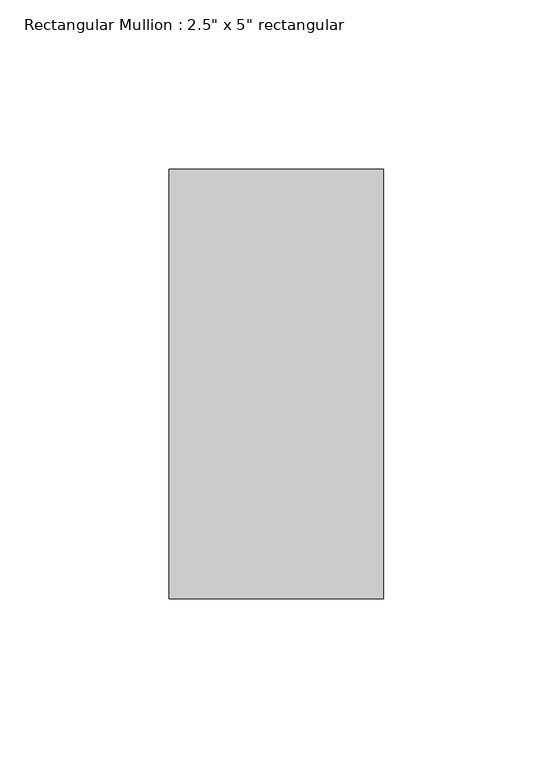
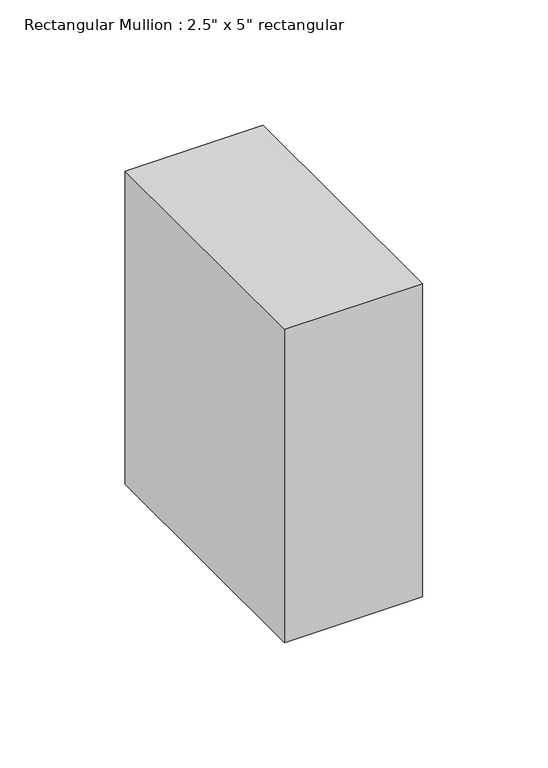
"""IFC4 building model written with IfcOpenShell, lengths in millimetres: member geometry."""

from ifc_helpers import new_model, si_unit, frame, origin, place, context, project, spatial, polyline, outline, extrude, source, transform, mapped, element, save


def member_876f8f00(model_context):
    return source(origin(), model_context, "Body", "SweptSolid", [
        extrude(outline(polyline([(0.0, 63.5), (0.0, -63.5), (-63.5, -63.5), (-63.5, 63.5), (0.0, 63.5)])), frame((0.0, 0.0, -152.4), z_axis=(0.0, 0.0, 1.0), x_axis=(1.0, 0.0, 0.0)), (0.0, 0.0, 1.0), 152.4),
    ])


if __name__ == "__main__":
    model = new_model("IFC4")
    model_context = context("Model", 3, world=origin())
    ifc_project = project(units=[si_unit("LENGTHUNIT", "METRE", prefix="MILLI")], contexts=[model_context])
    site = spatial("IfcSite", under=ifc_project)
    building = spatial("IfcBuilding", under=site)
    placement = place(None, origin())
    member_shape = member_876f8f00(model_context)
    element("IfcMember", 1, ObjectType="Rectangular Mullion : 2.5\" x 5\" rectangular", at=placement, inside=building, context=model_context, shape_type="MappedRepresentation", body=[
        mapped(member_shape, transform((0.0, 0.0, 0.0), x_axis=(1.0, 0.0, 0.0), y_axis=(0.0, 1.0, 0.0), z_axis=(0.0, 0.0, 1.0))),
    ])
    save(model, "model.ifc")

# Revit data of these elements
# Type "Rectangular Mullion : 2.5\" x 5\" rectangular"
#   built-in parameter 1007304 = 0.416667 (stored number, unit not read)
#   built-in parameter 1007301 = 0.104167 (stored number, unit not read)
#   built-in parameter 1007300 = 0.104167 (stored number, unit not read)
# Element 1 (IfcMember, "Rectangular Mullion : 2.5\" x 5\" rectangular")
#   Materials on its faces: "WINDOW FRAMING"
# Materials
#   "WINDOW FRAMING": class "Generic", colour RGB 120 120 120, transparency 0, Cost = 0
